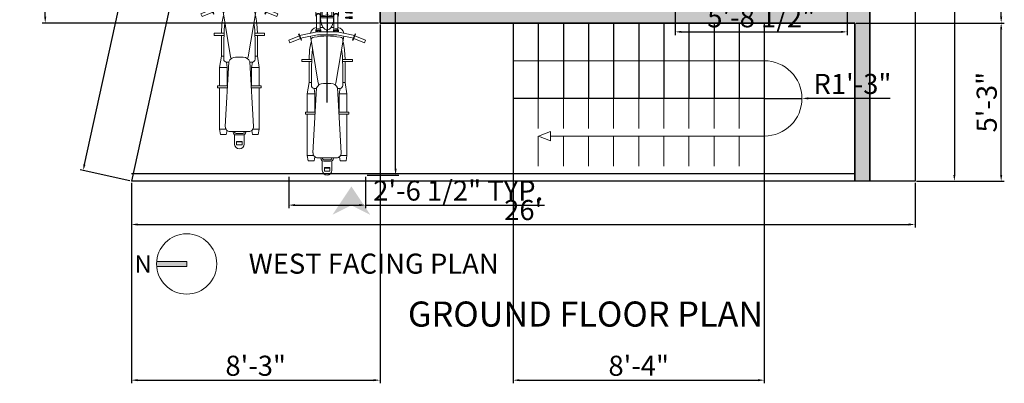
# Model space of a CAD drawing. Units: inches. Extents: x 2642 to 4124, y 1227 to 1973.
# Tile 1 of 7: x 3343 to 3735, y 1227 to 1372. Entities that reach past the tile are written whole.
import ezdxf

# ---------------------------------------------------------------- set-up
doc = ezdxf.new("R2010")
doc.units = ezdxf.units.IN
doc.linetypes.add('ACAD_ISO02W100', pattern=[15, 12, -3])
for name, color, linetype, lineweight in [('A-ANNO-DIMS', 2, 'Continuous', 18), ('A-ANNO-SYMB', 1, 'Continuous', 18), ('A-ANNO-TITL', 7, 'Continuous', 25), ('A-FLOR-STRS', 7, 'Continuous', 25), ('A-FLOR-STRS-OVHD', 7, 'ACAD_ISO02W100', 18), ('A-WALL', 7, 'Continuous', 35), ('A-WALL-PATT', 7, 'Continuous', 13), ('C-PRKG-VEHI', 8, 'Continuous', 18), ('C-PROP', 7, 'Continuous', 25)]:
    doc.layers.add(name, color=color, linetype=linetype, lineweight=lineweight)
doc.styles.get("Standard").update_dxf_attribs({"font": 'arial.ttf'})
doc.dimstyles.new('ISO-25', dxfattribs={"dimtxt": 8, "dimasz": 2.5, "dimexe": 1.25, "dimexo": 0.625, "dimtad": 1, "dimdec": 0, "dimlunit": 3, "dimtxsty": 'Standard', "dimcen": 2.5, "dimadec": 0, "dimazin": 0, "dimtfac": 1, "dimtdec": 0, "dimtmove": 0, "dimatfit": 3, "dimfxl": 1, "dimarcsym": 0})

# ---------------------------------------------------------------- blocks, each defined once
blk = doc.blocks.new('*D2')
at = {"layer": 'A-ANNO-DIMS', "color": 0, "lineweight": -2, "transparency": 16777216}
for p, q in [((3699.85, 1907.78), (3716.14, 1907.78)), ((3714.89, 1905.28), (3714.89, 1310.28)), ((3699.85, 1307.78), (3716.14, 1307.78))]:
    blk.add_line(p, q, dxfattribs=at)
at = {"layer": 'A-ANNO-DIMS', "color": 0, "transparency": 16777216}
for points in [[(3714.47, 1905.28), (3715.3, 1905.28), (3714.89, 1907.78)], [(3714.47, 1310.28), (3715.3, 1310.28), (3714.89, 1307.78)]]:
    blk.add_solid(points, dxfattribs=at)
at = {"layer": 'Defpoints', "color": 0, "transparency": 16777216}
for p in [(3699.22, 1907.78), (3699.22, 1307.78), (3714.89, 1307.78)]:
    blk.add_point(p, dxfattribs=at)
at = {"layer": 'A-ANNO-DIMS', "color": 0, "transparency": 16777216, "insert": (3710.18, 1607.78), "char_height": 8, "attachment_point": 5, "rotation": 90}
blk.add_mtext("50'", dxfattribs=at)
blk = doc.blocks.new('*D3')
at = {"layer": 'A-ANNO-DIMS', "color": 0, "lineweight": -2, "transparency": 16777216}
for p, q in [((3387.22, 1307.16), (3387.22, 1289.31)), ((3699.22, 1307.16), (3699.22, 1289.31)), ((3389.72, 1290.56), (3696.72, 1290.56))]:
    blk.add_line(p, q, dxfattribs=at)
at = {"layer": 'A-ANNO-DIMS', "color": 0, "transparency": 16777216}
for points in [[(3389.72, 1290.98), (3389.72, 1290.14), (3387.22, 1290.56)], [(3696.72, 1290.98), (3696.72, 1290.14), (3699.22, 1290.56)]]:
    blk.add_solid(points, dxfattribs=at)
at = {"layer": 'Defpoints', "color": 0, "transparency": 16777216}
for p in [(3387.22, 1307.78), (3699.22, 1307.78), (3699.22, 1290.56)]:
    blk.add_point(p, dxfattribs=at)
at = {"layer": 'A-ANNO-DIMS', "color": 0, "transparency": 16777216, "insert": (3543.22, 1295.27), "char_height": 8, "attachment_point": 5}
blk.add_mtext("26'", dxfattribs=at)
blk = doc.blocks.new('*D4')
at = {"layer": 'A-ANNO-DIMS', "color": 0, "lineweight": -2, "transparency": 16777216}
for p, q in [((3368.56, 1314.45), (3499.49, 1909.57)), ((3518.61, 1907.92), (3498.8, 1912.28)), ((3386.61, 1307.92), (3366.8, 1312.28))]:
    blk.add_line(p, q, dxfattribs=at)
at = {"layer": 'A-ANNO-DIMS', "color": 0, "transparency": 16777216}
for points in [[(3499.08, 1909.65), (3499.89, 1909.48), (3500.02, 1912.01)], [(3368.15, 1314.54), (3368.97, 1314.36), (3368.02, 1312.01)]]:
    blk.add_solid(points, dxfattribs=at)
at = {"layer": 'Defpoints', "color": 0, "transparency": 16777216}
for p in [(3500.02, 1912.01), (3519.22, 1907.78), (3387.22, 1307.78)]:
    blk.add_point(p, dxfattribs=at)
at = {"layer": 'A-ANNO-DIMS', "color": 0, "transparency": 16777216, "insert": (3429.42, 1613.02), "char_height": 8, "attachment_point": 5, "rotation": 77.5926}
blk.add_mtext('51\'-2"', dxfattribs=at)
blk = doc.blocks.new('BIKE')
for p, q in [((34846.04, 15170.34), (34846.04, 15168.87)), ((34847.86, 15170.34), (34847.86, 15168.87)), ((34845.81, 15167.86), (34845.81, 15160.7)), ((34845.81, 15167.86), (34845.81, 15160.7)), ((34848.09, 15167.86), (34848.09, 15160.7)), ((34844.29, 15164.4), (34844.29, 15160.81)), ((34845.43, 15164.4), (34845.43, 15160.81)), ((34845.43, 15164.1), (34845.81, 15164.1)), ((34845.43, 15163.85), (34845.81, 15163.85)), ((34848.47, 15164.1), (34848.09, 15164.1)), ((34848.47, 15163.85), (34848.09, 15163.85)), ((34848.47, 15164.4), (34848.47, 15160.81)), ((34849.61, 15164.4), (34849.61, 15160.81)), ((34844.41, 15160.81), (34844.41, 15157.43)), ((34845.32, 15160.81), (34845.32, 15157.43)), ((34848.58, 15160.81), (34848.58, 15157.43)), ((34849.5, 15160.81), (34849.5, 15157.43)), ((34848.51, 15160.53), (34845.39, 15160.53)), ((34845.39, 15160.23), (34845.39, 15160.53)), ((34845.39, 15160.23), (34845.39, 15160.53)), ((34848.51, 15160.23), (34845.39, 15160.23)), ((34848.51, 15160.23), (34848.51, 15160.53)), ((34840.19, 15156.35), (34840.3, 15156.39)), ((34840.19, 15156.35), (34840.8, 15154.88)), ((34840.3, 15156.39), (34840.9, 15154.92)), ((34840.47, 15155.97), (34840.8, 15156.11)), ((34840.8, 15156.11), (34844.56, 15156.88)), ((34841, 15155.45), (34844.63, 15156.2)), ((34844.29, 15156.87), (34844.29, 15157.17)), ((34844.41, 15156.87), (34844.41, 15156.85)), ((34844.56, 15156.88), (34846.95, 15156.88)), ((34844.63, 15156.2), (34846.95, 15156.2)), ((34845.32, 15157.92), (34846.04, 15157.92)), ((34845.43, 15156.87), (34845.43, 15157.17)), ((34849.34, 15156.88), (34846.95, 15156.88)), ((34849.27, 15156.2), (34846.95, 15156.2)), ((34848.58, 15157.92), (34847.87, 15157.92)), ((34848.47, 15156.87), (34848.47, 15157.17)), ((34852.9, 15155.45), (34849.27, 15156.2)), ((34853.1, 15156.11), (34849.34, 15156.88)), ((34849.5, 15156.87), (34849.5, 15156.85)), ((34849.61, 15156.87), (34849.61, 15157.17)), ((34853.6, 15156.39), (34853, 15154.92)), ((34853.71, 15156.35), (34853.1, 15154.88)), ((34853.43, 15155.97), (34853.1, 15156.11)), ((34853.71, 15156.35), (34853.6, 15156.39)), ((34837.84, 15154.89), (34840.37, 15155.93)), ((34837.84, 15154.89), (34838.1, 15154.26)), ((34838.1, 15154.26), (34840.63, 15155.3)), ((34840.73, 15155.34), (34841, 15155.45)), ((34840.8, 15154.88), (34840.9, 15154.92)), ((34842.8, 15152.59), (34843.06, 15154.2)), ((34844.86, 15144.72), (34843.01, 15155.87)), ((34843.06, 15154.2), (34843.22, 15154.58)), ((34849.05, 15144.72), (34850.89, 15155.87)), ((34850.84, 15154.2), (34850.68, 15154.58)), ((34851.1, 15152.59), (34850.84, 15154.2)), ((34853.17, 15155.34), (34852.9, 15155.45)), ((34853.1, 15154.88), (34853, 15154.92)), ((34855.81, 15154.26), (34853.28, 15155.3)), ((34856.07, 15154.89), (34853.54, 15155.93)), ((34856.07, 15154.89), (34855.81, 15154.26)), ((34842.7, 15150.31), (34842.8, 15152.59)), ((34843.33, 15151.09), (34843.52, 15152.8)), ((34850.57, 15151.09), (34850.38, 15152.8)), ((34851.2, 15150.31), (34851.1, 15152.59)), ((34840.97, 15150.31), (34843.3, 15150.31)), ((34840.97, 15149.81), (34840.97, 15150.31)), ((34843.29, 15149.81), (34840.97, 15149.81)), ((34842.7, 15144.87), (34842.7, 15149.81)), ((34843.23, 15147.75), (34843.33, 15151.09)), ((34850.67, 15147.75), (34850.57, 15151.09)), ((34852.93, 15150.31), (34850.6, 15150.31)), ((34850.61, 15149.81), (34852.93, 15149.81)), ((34851.2, 15144.87), (34851.2, 15149.81)), ((34852.93, 15149.81), (34852.93, 15150.31)), ((34843.23, 15144.15), (34843.23, 15147.75)), ((34850.67, 15144.15), (34850.67, 15147.75)), ((34842.7, 15144.87), (34842.25, 15142.19)), ((34842.7, 15144.87), (34843.23, 15144.87)), ((34847.85, 15144.64), (34846.06, 15144.64)), ((34851.2, 15144.87), (34850.67, 15144.87)), ((34851.2, 15144.87), (34851.65, 15142.19)), ((34842.25, 15142.19), (34844.07, 15142.19)), ((34842.25, 15137.82), (34842.25, 15142.19)), ((34844.46, 15143.56), (34843.6, 15128.2)), ((34843.85, 15143.46), (34844.07, 15142.19)), ((34843.91, 15143.46), (34844.46, 15143.46)), ((34844.07, 15137.82), (34844.07, 15142.19)), ((34849.44, 15143.56), (34850.3, 15128.2)), ((34849.99, 15143.46), (34849.44, 15143.46)), ((34850.05, 15143.46), (34849.83, 15142.19)), ((34851.65, 15142.19), (34849.83, 15142.19)), ((34849.83, 15137.82), (34849.83, 15142.19)), ((34851.65, 15137.82), (34851.65, 15142.19)), ((34841.79, 15137.82), (34844.14, 15137.82)), ((34841.79, 15137.33), (34841.79, 15137.82)), ((34852.11, 15137.82), (34849.76, 15137.82)), ((34852.11, 15137.33), (34852.11, 15137.82)), ((34844.11, 15137.33), (34841.79, 15137.33)), ((34842.25, 15127.57), (34842.25, 15137.33)), ((34844.07, 15136.55), (34844.07, 15137.33)), ((34849.79, 15137.33), (34852.11, 15137.33)), ((34849.83, 15136.55), (34849.83, 15137.33)), ((34851.65, 15127.57), (34851.65, 15137.33)), ((34842.25, 15127.57), (34843.75, 15127.57)), ((34842.25, 15127.57), (34842.48, 15126.27)), ((34842.48, 15126.27), (34843.84, 15126.27)), ((34844.02, 15127.25), (34843.84, 15126.27)), ((34849.16, 15126.99), (34844.74, 15126.99)), ((34845.47, 15126.99), (34845.47, 15126.88)), ((34845.81, 15126.99), (34845.81, 15126.88)), ((34845.81, 15126.29), (34845.81, 15124.03)), ((34847.75, 15126.54), (34846.15, 15126.54)), ((34847.75, 15126.2), (34846.15, 15126.2)), ((34848.09, 15126.99), (34848.09, 15126.88)), ((34848.09, 15126.29), (34848.09, 15124.03)), ((34848.43, 15126.99), (34848.43, 15126.88)), ((34849.89, 15127.25), (34850.06, 15126.27)), ((34851.43, 15126.27), (34850.06, 15126.27)), ((34851.65, 15127.57), (34850.15, 15127.57)), ((34851.65, 15127.57), (34851.43, 15126.27)), ((34846.29, 15123.82), (34846.29, 15124.66)), ((34846.29, 15124.66), (34847.61, 15124.66)), ((34846.29, 15124.55), (34847.61, 15124.55)), ((34847.61, 15123.82), (34846.29, 15123.82)), ((34847.61, 15124.66), (34847.61, 15123.82))]:
    blk.add_line(p, q)
for points in [[(34845.81, 15167.86, -0.068977), (34845.9, 15168.53, -0.081012), (34846.15, 15169.05, -0.107014), (34846.54, 15169.42, -0.137239), (34846.95, 15169.53, -0.137239), (34847.36, 15169.42, -0.107014), (34847.76, 15169.05, -0.081012), (34848, 15168.53, -0.068977), (34848.09, 15167.86, -0.068977)], [(34845.43, 15164.4, 0.125099), (34845.39, 15164.56, 0.105827), (34845.27, 15164.71, 0.086577), (34845.09, 15164.8, 0.0766), (34844.86, 15164.84, 0.0766), (34844.64, 15164.8, 0.086577), (34844.46, 15164.71, 0.105827), (34844.33, 15164.56, 0.125099), (34844.29, 15164.4, 0.125099)], [(34848.47, 15164.4, -0.125099), (34848.51, 15164.56, -0.105827), (34848.64, 15164.71, -0.086577), (34848.82, 15164.8, -0.0766), (34849.04, 15164.84, -0.0766), (34849.26, 15164.8, -0.086577), (34849.44, 15164.71, -0.105827), (34849.57, 15164.56, -0.125099), (34849.61, 15164.4, -0.125099)], [(34845.32, 15160.55, 0.067261), (34845.39, 15160.65, 0.125099), (34845.43, 15160.81, 0.125099), (34845.39, 15160.97, 0.105827), (34845.27, 15161.12, 0.086577), (34845.09, 15161.21, 0.0766), (34844.86, 15161.25, 0.0766), (34844.64, 15161.21, 0.086577), (34844.46, 15161.12, 0.105827), (34844.33, 15160.97, 0.125099), (34844.29, 15160.81, 0.125099)], [(34844.29, 15160.81, 0.125099), (34844.33, 15160.65, 0.067261), (34844.41, 15160.55, 0.086577)], [(34845.32, 15160.81, 0.125099), (34845.29, 15160.92, 0.105827), (34845.2, 15161.03, 0.086577), (34845.05, 15161.1, 0.0766), (34844.86, 15161.13, 0.0766), (34844.67, 15161.1, 0.086577), (34844.53, 15161.03, 0.105827), (34844.43, 15160.92, 0.125099), (34844.41, 15160.81, 0.125099)], [(34848.58, 15160.55, -0.067261), (34848.51, 15160.65, -0.125099), (34848.47, 15160.81, -0.125099), (34848.51, 15160.97, -0.105827), (34848.64, 15161.12, -0.086577), (34848.82, 15161.21, -0.0766), (34849.04, 15161.25, -0.0766), (34849.26, 15161.21, -0.086577), (34849.44, 15161.12, -0.105827), (34849.57, 15160.97, -0.125099), (34849.61, 15160.81, -0.125099)], [(34848.58, 15160.81, -0.125099), (34848.61, 15160.92, -0.105827), (34848.71, 15161.03, -0.086577), (34848.85, 15161.1, -0.0766), (34849.04, 15161.13, -0.0766), (34849.23, 15161.1, -0.086577), (34849.37, 15161.03, -0.105827), (34849.47, 15160.92, -0.125099), (34849.5, 15160.81, -0.125099)], [(34849.61, 15160.81, -0.125099), (34849.57, 15160.65, -0.067261), (34849.5, 15160.55, -0.086577)], [(34846.95, 15157.37, -0.163989), (34846.41, 15157.55, -0.105862), (34845.85, 15158.21, -0.069323), (34845.52, 15159.08, -0.055531), (34845.39, 15160.23, -0.055531)], [(34848.51, 15160.23, -0.055531), (34848.38, 15159.08, -0.069323), (34848.06, 15158.21, -0.105862), (34847.49, 15157.55, -0.163989), (34846.95, 15157.37, -0.163989)], [(34845.43, 15157.17, 0.125099), (34845.39, 15157.33, 0.105827), (34845.27, 15157.48, 0.086577), (34845.09, 15157.57, 0.0766), (34844.86, 15157.6, 0.0766), (34844.64, 15157.57, 0.086577), (34844.46, 15157.48, 0.105827), (34844.33, 15157.33, 0.125099), (34844.29, 15157.17, 0.125099)], [(34845.43, 15156.88, 0.117252), (34845.39, 15157.03, 0.105827), (34845.27, 15157.18, 0.086577), (34845.09, 15157.27, 0.0766), (34844.86, 15157.31, 0.0766), (34844.64, 15157.27, 0.086577), (34844.46, 15157.18, 0.105827), (34844.33, 15157.03, 0.125099), (34844.29, 15156.87, 0.125099)], [(34844.29, 15156.87, 0.032819), (34844.3, 15156.83, 0.067261)], [(34845.32, 15156.88, 0.113202), (34845.29, 15156.98, 0.105827), (34845.2, 15157.09, 0.086577), (34845.05, 15157.16, 0.0766), (34844.86, 15157.19, 0.0766), (34844.67, 15157.16, 0.086577), (34844.53, 15157.09, 0.105827), (34844.43, 15156.98, 0.125099), (34844.41, 15156.87, 0.125099)], [(34848.47, 15157.17, -0.125099), (34848.51, 15157.33, -0.105827), (34848.64, 15157.48, -0.086577), (34848.82, 15157.57, -0.0766), (34849.04, 15157.6, -0.0766), (34849.26, 15157.57, -0.086577), (34849.44, 15157.48, -0.105827), (34849.57, 15157.33, -0.125099), (34849.61, 15157.17, -0.125099)], [(34848.47, 15156.88, -0.117252), (34848.51, 15157.03, -0.105827), (34848.64, 15157.18, -0.086577), (34848.82, 15157.27, -0.0766), (34849.04, 15157.31, -0.0766), (34849.26, 15157.27, -0.086577), (34849.44, 15157.18, -0.105827), (34849.57, 15157.03, -0.125099), (34849.61, 15156.87, -0.125099)], [(34848.58, 15156.88, -0.113202), (34848.61, 15156.98, -0.105827), (34848.71, 15157.09, -0.086577), (34848.85, 15157.16, -0.0766), (34849.04, 15157.19, -0.0766), (34849.23, 15157.16, -0.086577), (34849.37, 15157.09, -0.105827), (34849.47, 15156.98, -0.125099), (34849.5, 15156.87, -0.125099)], [(34849.61, 15156.87, -0.032819), (34849.61, 15156.83, -0.067261)]]:
    blk.add_lwpolyline(points, format="xyb")
for centre, radius, start, end in [((34846.95, 15157.24), 3.64, 64.5882, 115.4118), ((34844.55, 15156.32), 1.59, 95.2207, 171.678), ((34849.35, 15156.32), 1.59, 8.322, 84.7793), ((34843.86, 15154.92), 0.684, 90, 189.3898), ((34846.95, 15140.12), 15.79, 78.7129, 101.2871), ((34850.04, 15154.92), 0.684, 350.6102, 90), ((34846, 15143), 1.64, 88.1125, 159.9264), ((34845.53, 15144.83), 0.684, 189.3898, 226.4877), ((34847.9, 15143), 1.64, 20.0736, 91.8875), ((34848.37, 15144.83), 0.684, 313.5123, 350.6102), ((34843.91, 15144.15), 0.684, 180, 270), ((34849.99, 15144.15), 0.684, 270, 0), ((34844.74, 15128.13), 1.14, 176.7865, 270), ((34849.16, 15128.13), 1.14, 270, 3.2135), ((34846.15, 15126.88), 0.684, 180, 270), ((34846.15, 15126.88), 0.342, 180, 270), ((34847.75, 15126.88), 0.684, 270, 0), ((34847.75, 15126.88), 0.342, 270, 0), ((34846.95, 15124.03), 1.14, 180, 0)]:
    blk.add_arc(centre, radius, start, end)
blk = doc.blocks.new('*D48')
at = {"layer": 'A-ANNO-DIMS', "color": 0, "lineweight": -2, "transparency": 16777216}
for p, q in [((3492.41, 1389.89), (3492.41, 1489.27)), ((3481.09, 1389.89), (3493.66, 1389.89)), ((3492.41, 1312.73), (3492.41, 1387.39)), ((3481.09, 1310.23), (3493.66, 1310.23))]:
    blk.add_line(p, q, dxfattribs=at)
at = {"layer": 'A-ANNO-DIMS', "color": 0, "transparency": 16777216}
for points in [[(3492, 1387.39), (3492.83, 1387.39), (3492.41, 1389.89)], [(3492, 1312.73), (3492.83, 1312.73), (3492.41, 1310.23)]]:
    blk.add_solid(points, dxfattribs=at)
at = {"layer": 'Defpoints', "color": 0, "transparency": 16777216}
for p in [(3480.46, 1389.89), (3492.41, 1389.89), (3480.46, 1310.23)]:
    blk.add_point(p, dxfattribs=at)
at = {"layer": 'A-ANNO-DIMS', "color": 0, "transparency": 16777216, "insert": (3487.65, 1440.83), "char_height": 8, "attachment_point": 5, "rotation": 90}
blk.add_mtext('BIKE 6\'-7 1/2" TYP.', dxfattribs=at)
blk = doc.blocks.new('*D49')
at = {"layer": 'A-ANNO-DIMS', "color": 0, "lineweight": -2, "transparency": 16777216}
for p, q in [((3449.86, 1309.6), (3449.86, 1297.03)), ((3480.46, 1309.6), (3480.46, 1297.03)), ((3452.36, 1298.28), (3477.96, 1298.28)), ((3480.46, 1298.28), (3551.75, 1298.28))]:
    blk.add_line(p, q, dxfattribs=at)
at = {"layer": 'A-ANNO-DIMS', "color": 0, "transparency": 16777216}
for points in [[(3452.36, 1298.69), (3452.36, 1297.86), (3449.86, 1298.28)], [(3477.96, 1298.69), (3477.96, 1297.86), (3480.46, 1298.28)]]:
    blk.add_solid(points, dxfattribs=at)
at = {"layer": 'Defpoints', "color": 0, "transparency": 16777216}
for p in [(3449.86, 1310.23), (3480.46, 1310.23), (3480.46, 1298.28)]:
    blk.add_point(p, dxfattribs=at)
at = {"layer": 'A-ANNO-DIMS', "color": 0, "transparency": 16777216, "insert": (3517.36, 1303.04), "char_height": 8, "attachment_point": 5}
blk.add_mtext('2\'-6 1/2" TYP.', dxfattribs=at)
blk = doc.blocks.new('*D55')
at = {"layer": 'A-ANNO-DIMS', "color": 0, "lineweight": -2, "transparency": 16777216}
for p, q in [((3603.75, 1379.31), (3603.75, 1366.03)), ((3672.22, 1379.31), (3672.22, 1366.03)), ((3606.25, 1367.28), (3669.72, 1367.28))]:
    blk.add_line(p, q, dxfattribs=at)
at = {"layer": 'A-ANNO-DIMS', "color": 0, "transparency": 16777216}
for points in [[(3606.25, 1367.7), (3606.25, 1366.87), (3603.75, 1367.28)], [(3669.72, 1367.7), (3669.72, 1366.87), (3672.22, 1367.28)]]:
    blk.add_solid(points, dxfattribs=at)
at = {"layer": 'Defpoints', "color": 0, "transparency": 16777216}
for p in [(3603.75, 1379.93), (3672.22, 1379.93), (3672.22, 1367.28)]:
    blk.add_point(p, dxfattribs=at)
at = {"layer": 'A-ANNO-DIMS', "color": 0, "transparency": 16777216, "insert": (3637.99, 1372.04), "char_height": 8, "attachment_point": 5}
blk.add_mtext('5\'-8 1/2"', dxfattribs=at)
blk = doc.blocks.new('*D68')
at = {"layer": 'A-ANNO-DIMS', "color": 0, "lineweight": -2, "transparency": 16777216}
for p, q in [((3675.85, 1370.78), (3734.77, 1370.78)), ((3733.52, 1310.28), (3733.52, 1368.28)), ((3699.85, 1307.78), (3734.77, 1307.78))]:
    blk.add_line(p, q, dxfattribs=at)
at = {"layer": 'A-ANNO-DIMS', "color": 0, "transparency": 16777216}
for points in [[(3733.11, 1368.28), (3733.94, 1368.28), (3733.52, 1370.78)], [(3733.11, 1310.28), (3733.94, 1310.28), (3733.52, 1307.78)]]:
    blk.add_solid(points, dxfattribs=at)
at = {"layer": 'Defpoints', "color": 0, "transparency": 16777216}
for p in [(3675.22, 1370.78), (3733.52, 1370.78), (3699.22, 1307.78)]:
    blk.add_point(p, dxfattribs=at)
at = {"layer": 'A-ANNO-DIMS', "color": 0, "transparency": 16777216, "insert": (3728.81, 1339.28), "char_height": 8, "attachment_point": 5, "rotation": 90}
blk.add_mtext('5\'-3"', dxfattribs=at)
blk = doc.blocks.new('*D69')
at = {"layer": 'A-ANNO-DIMS', "color": 0, "lineweight": -2, "transparency": 16777216}
for p, q in [((3486.22, 1370.16), (3486.22, 1227.29)), ((3387.22, 1307.16), (3387.22, 1227.29)), ((3389.72, 1228.54), (3483.72, 1228.54))]:
    blk.add_line(p, q, dxfattribs=at)
at = {"layer": 'A-ANNO-DIMS', "color": 0, "transparency": 16777216}
for points in [[(3389.72, 1228.96), (3389.72, 1228.12), (3387.22, 1228.54)], [(3483.72, 1228.96), (3483.72, 1228.12), (3486.22, 1228.54)]]:
    blk.add_solid(points, dxfattribs=at)
at = {"layer": 'Defpoints', "color": 0, "transparency": 16777216}
for p in [(3486.22, 1370.78), (3387.22, 1307.78), (3486.22, 1228.54)]:
    blk.add_point(p, dxfattribs=at)
at = {"layer": 'A-ANNO-DIMS', "color": 0, "transparency": 16777216, "insert": (3436.72, 1233.25), "char_height": 8, "attachment_point": 5}
blk.add_mtext('8\'-3"', dxfattribs=at)
blk = doc.blocks.new('*D72')
at = {"layer": 'A-ANNO-DIMS', "color": 0, "lineweight": -2, "transparency": 16777216}
for p, q in [((3485.6, 1508.78), (3351.67, 1508.78)), ((3352.92, 1373.28), (3352.92, 1506.28)), ((3485.6, 1370.78), (3351.67, 1370.78))]:
    blk.add_line(p, q, dxfattribs=at)
at = {"layer": 'A-ANNO-DIMS', "color": 0, "transparency": 16777216}
for points in [[(3352.51, 1506.28), (3353.34, 1506.28), (3352.92, 1508.78)], [(3352.51, 1373.28), (3353.34, 1373.28), (3352.92, 1370.78)]]:
    blk.add_solid(points, dxfattribs=at)
at = {"layer": 'Defpoints', "color": 0, "transparency": 16777216}
for p in [(3352.92, 1508.78), (3486.22, 1508.78), (3486.22, 1370.78)]:
    blk.add_point(p, dxfattribs=at)
at = {"layer": 'A-ANNO-DIMS', "color": 0, "transparency": 16777216, "insert": (3348.21, 1439.78), "char_height": 8, "attachment_point": 5, "rotation": 90}
blk.add_mtext('11\'-6"', dxfattribs=at)
blk = doc.blocks.new('*D73')
at = {"layer": 'A-ANNO-DIMS', "color": 0, "lineweight": -2, "transparency": 16777216}
for p, q in [((3539.22, 1370.16), (3539.22, 1227.29)), ((3639.22, 1370.16), (3639.22, 1227.29)), ((3541.72, 1228.54), (3636.72, 1228.54))]:
    blk.add_line(p, q, dxfattribs=at)
at = {"layer": 'A-ANNO-DIMS', "color": 0, "transparency": 16777216}
for points in [[(3541.72, 1228.96), (3541.72, 1228.12), (3539.22, 1228.54)], [(3636.72, 1228.96), (3636.72, 1228.12), (3639.22, 1228.54)]]:
    blk.add_solid(points, dxfattribs=at)
at = {"layer": 'Defpoints', "color": 0, "transparency": 16777216}
for p in [(3539.22, 1370.78), (3639.22, 1370.78), (3639.22, 1228.54)]:
    blk.add_point(p, dxfattribs=at)
at = {"layer": 'A-ANNO-DIMS', "color": 0, "transparency": 16777216, "insert": (3589.22, 1233.25), "char_height": 8, "attachment_point": 5}
blk.add_mtext('8\'-4"', dxfattribs=at)
blk = doc.blocks.new('*D74')
at = {"layer": 'A-ANNO-DIMS', "color": 0, "lineweight": -2, "transparency": 16777216}
for p, q in [((3681.85, 1427.78), (3734.77, 1427.78)), ((3733.52, 1373.28), (3733.52, 1425.28)), ((3675.85, 1370.78), (3734.77, 1370.78))]:
    blk.add_line(p, q, dxfattribs=at)
at = {"layer": 'A-ANNO-DIMS', "color": 0, "transparency": 16777216}
for points in [[(3733.11, 1425.28), (3733.94, 1425.28), (3733.52, 1427.78)], [(3733.11, 1373.28), (3733.94, 1373.28), (3733.52, 1370.78)]]:
    blk.add_solid(points, dxfattribs=at)
at = {"layer": 'Defpoints', "color": 0, "transparency": 16777216}
for p in [(3681.22, 1427.78), (3733.52, 1427.78), (3675.22, 1370.78)]:
    blk.add_point(p, dxfattribs=at)
at = {"layer": 'A-ANNO-DIMS', "color": 0, "transparency": 16777216, "insert": (3728.81, 1399.28), "char_height": 8, "attachment_point": 5, "rotation": 90}
blk.add_mtext('4\'-9"', dxfattribs=at)
blk = doc.blocks.new('*D82')
at = {"layer": 'A-ANNO-DIMS', "color": 0, "lineweight": -2, "transparency": 16777216}
for p, q in [((3639.22, 1340.78), (3654.22, 1340.78)), ((3689.39, 1340.78), (3656.72, 1340.78))]:
    blk.add_line(p, q, dxfattribs=at)
at = {"layer": 'A-ANNO-DIMS', "color": 0, "transparency": 16777216}
blk.add_solid([(3656.72, 1341.2), (3656.72, 1340.37), (3654.22, 1340.78)], dxfattribs=at)
at = {"layer": 'Defpoints', "color": 0, "transparency": 16777216}
for p in [(3639.22, 1340.78), (3654.22, 1340.78)]:
    blk.add_point(p, dxfattribs=at)
at = {"layer": 'A-ANNO-DIMS', "color": 0, "transparency": 16777216, "insert": (3674.31, 1345.5), "char_height": 8, "attachment_point": 5, "rotation": 359.9998}
blk.add_mtext('R1\'-3"', dxfattribs=at)
blk = doc.blocks.new('*D84')
at = {"layer": 'A-ANNO-DIMS', "color": 0, "lineweight": -2, "transparency": 16777216}
for p, q in [((3465.16, 1436.8), (3465.16, 1368.17)), ((3465.16, 1339.16), (3465.16, 1365.67))]:
    blk.add_line(p, q, dxfattribs=at)
at = {"layer": 'A-ANNO-DIMS', "color": 0, "transparency": 16777216}
blk.add_solid([(3465.58, 1368.17), (3464.74, 1368.17), (3465.16, 1365.67)], dxfattribs=at)
at = {"layer": 'Defpoints', "color": 0, "transparency": 16777216}
for p in [(3465.16, 1365.67), (3465.16, 1339.16)]:
    blk.add_point(p, dxfattribs=at)
at = {"layer": 'A-ANNO-DIMS', "color": 0, "transparency": 16777216, "insert": (3469.92, 1403.74), "char_height": 8, "attachment_point": 5, "rotation": 270.0011}
blk.add_mtext('2X R2\'-2 1/2"', dxfattribs=at)

msp = doc.modelspace()

# ---------------------------------------------------------------- hatches: boundary and pattern name
at = {"layer": 'A-ANNO-SYMB'}
h = msp.add_hatch(color=256, dxfattribs=at)
h.dxf.hatch_style = 1
h.paths.add_polyline_path([(3474.82, 1305.73), (3467.27, 1294.41), (3474.82, 1298.18), (3482.37, 1294.41)])
h = msp.add_hatch(color=256, dxfattribs=at)
h.dxf.hatch_style = 1
h.paths.add_polyline_path([(3409.24, 1275.84), (3409.24, 1273.84), (3397.28, 1273.84, -0.020861), (3397.24, 1274.84, -0.020861), (3397.28, 1275.84)])
at = {"layer": 'A-WALL-PATT'}
h = msp.add_hatch(color=256, dxfattribs=at)
h.dxf.hatch_style = 1
h.paths.add_polyline_path([(3552.22, 1505.78), (3495.22, 1505.78), (3495.22, 1508.78), (3492.22, 1508.78), (3486.22, 1508.78), (3486.22, 1415.78), (3495.22, 1415.78), (3495.22, 1499.78), (3543.22, 1499.78), (3543.22, 1457.78), (3549.22, 1457.78), (3549.22, 1499.78), (3552.19, 1499.78), (3552.19, 1499.78)])
h.paths.add_polyline_path([(3681.22, 1427.78), (3672.22, 1427.78), (3672.22, 1395.07), (3672.22, 1379.78), (3549.22, 1379.78), (3549.22, 1427.78), (3543.22, 1427.78), (3543.22, 1379.78), (3495.22, 1379.78), (3495.22, 1391.78), (3486.22, 1391.78), (3486.22, 1370.78), (3675.22, 1370.78), (3675.22, 1307.78), (3681.22, 1307.78)])
h.paths.add_polyline_path([(3681.22, 1517.78), (3672.22, 1517.78), (3672.22, 1505.78), (3640.73, 1505.78), (3588.22, 1505.78), (3588.22, 1499.78), (3672.22, 1499.78), (3672.22, 1475.78), (3681.22, 1475.78)])
h.paths.add_polyline_path([(3681.22, 1638.12), (3672.22, 1638.12), (3672.22, 1625.78), (3681.22, 1625.78)])
h.paths.add_polyline_path([(3681.22, 1553.78), (3672.22, 1553.78), (3672.22, 1541.78), (3681.22, 1541.78)])
h.paths.add_polyline_path([(3528.22, 1844.78), (3552.22, 1844.78), (3552.22, 1847.78), (3552.22, 1853.78), (3519.22, 1853.78), (3519.22, 1682.78), (3486.22, 1682.78), (3486.22, 1548.78), (3492.22, 1548.78), (3495.22, 1548.78), (3495.22, 1673.78), (3528.22, 1673.78)])
h.paths.add_polyline_path([(3681.22, 1865.78), (3675.22, 1865.78), (3675.22, 1853.78), (3615.22, 1853.78), (3615.22, 1856.78), (3609.22, 1856.78), (3609.22, 1853.78), (3582.22, 1853.78), (3582.22, 1847.78), (3582.22, 1844.78), (3672.22, 1844.78), (3672.22, 1823.67), (3681.22, 1823.67)])
h.paths.add_polyline_path([(3681.22, 1907.78), (3519.22, 1907.78), (3519.22, 1901.78), (3540.68, 1901.78), (3609.22, 1901.78), (3609.22, 1886.78), (3615.22, 1886.78), (3615.22, 1901.78), (3675.22, 1901.78), (3675.22, 1889.78), (3681.22, 1889.78)])
h.paths.add_polyline_path([(3681.22, 1775.67), (3672.22, 1775.67), (3672.22, 1742.87), (3681.22, 1742.87)])
h.paths.add_polyline_path([(3681.22, 1694.87), (3672.22, 1694.87), (3672.22, 1682.78), (3600.22, 1682.78), (3600.22, 1673.78), (3672.22, 1673.78), (3672.22, 1662.12), (3681.22, 1662.12)])

# ---------------------------------------------------------------- linework, layer by layer
at = {"layer": 'A-ANNO-SYMB'}
for p, q in [((3409.24, 1275.84), (3397.28, 1275.84)), ((3409.24, 1273.84), (3409.24, 1275.84)), ((3397.24, 1273.84), (3409.24, 1273.84))]:
    msp.add_line(p, q, dxfattribs=at)
for points in [[(3539.22, 1355.78), (3639.22, 1355.78)], [(3554.08, 1325.78), (3639.22, 1325.78)]]:
    msp.add_lwpolyline(points, dxfattribs=at)
msp.add_lwpolyline([(3549.32, 1325.78), (3554.08, 1323.91), (3554.08, 1327.65)], close=True, dxfattribs=at)
msp.add_circle((3409.24, 1274.84), 12, dxfattribs=at)
msp.add_arc((3639.22, 1340.78), 15, 270, 90, dxfattribs=at)
at = {"layer": 'A-FLOR-STRS'}
for p, q in [((3539.22, 1370.78), (3539.22, 1340.78)), ((3549.22, 1370.78), (3549.22, 1340.78)), ((3559.22, 1370.78), (3559.22, 1340.78)), ((3569.22, 1370.78), (3569.22, 1340.78)), ((3579.22, 1370.78), (3579.22, 1340.78)), ((3589.22, 1370.78), (3589.22, 1340.78)), ((3599.22, 1370.78), (3599.22, 1340.78)), ((3609.22, 1370.78), (3609.22, 1340.78)), ((3619.22, 1370.78), (3619.22, 1340.78)), ((3629.22, 1370.78), (3629.22, 1340.78)), ((3639.22, 1370.78), (3639.22, 1310.78)), ((3639.22, 1340.78), (3539.22, 1340.78))]:
    msp.add_line(p, q, dxfattribs=at)
at = {"layer": 'A-FLOR-STRS-OVHD'}
for p, q in [((3549.22, 1340.78), (3549.22, 1310.78)), ((3559.22, 1340.78), (3559.22, 1310.78)), ((3569.22, 1340.78), (3569.22, 1310.78)), ((3579.22, 1340.78), (3579.22, 1310.78)), ((3589.22, 1340.78), (3589.22, 1310.78)), ((3599.22, 1340.78), (3599.22, 1310.78)), ((3609.22, 1340.78), (3609.22, 1310.78)), ((3619.22, 1340.78), (3619.22, 1310.78)), ((3629.22, 1340.78), (3629.22, 1310.78))]:
    msp.add_line(p, q, dxfattribs=at)
at = {"layer": 'A-WALL'}
for p, q in [((3681.22, 1907.78), (3681.22, 1307.78)), ((3486.22, 1508.78), (3486.22, 1370.78)), ((3675.22, 1370.78), (3486.22, 1370.78)), ((3675.22, 1370.78), (3675.22, 1307.78))]:
    msp.add_line(p, q, dxfattribs=at)
at = {"layer": 'C-PROP'}
for p, q in [((3519.22, 1907.78), (3387.22, 1307.78)), ((3699.22, 1907.78), (3699.22, 1307.78)), ((3675.22, 1310.78), (3387.22, 1310.78)), ((3699.22, 1307.78), (3387.22, 1307.78))]:
    msp.add_line(p, q, dxfattribs=at)

# ---------------------------------------------------------------- block references
at = {"layer": 'C-PRKG-VEHI', "xscale": 1.67889555227424, "yscale": 1.67889555227424, "zscale": 1.67889555227424}
for p in [(-55074.15, -24069.06), (-55039.23, -24079.53)]:
    msp.add_blockref('BIKE', p, dxfattribs=at)

# ---------------------------------------------------------------- texts
at = {"layer": 'A-ANNO-SYMB'}
msp.add_text('N', height=6.9, dxfattribs=at).set_placement((3388.5, 1271.31))
at = {"layer": 'A-ANNO-TITL', "attachment_point": 1}
for s, insert, char_height in [('{\\fTimes New Roman|b0|i0|c0|p18;WEST FACING PLAN}', (3433.93, 1278.96), 8), ('{\\fTimes New Roman|b0|i0|c0|p18;GROUND FLOOR PLAN}', (3497.33, 1259.88), 10)]:
    msp.add_mtext_dynamic_manual_height_columns(s, width=196.2607, gutter_width=12.5, heights=[0], dxfattribs=dict(at, insert=insert, char_height=char_height))

# ---------------------------------------------------------------- dimensions: what is measured, and where the dimension line sits
at = {"layer": 'A-ANNO-DIMS'}
dim = msp.add_aligned_dim(p1=(3387.22, 1307.78), p2=(3519.22, 1907.78), distance=19.66, dimstyle='ISO-25', override={"dimclrd": 0, "dimclre": 0, "dimclrt": 0}, dxfattribs=at)
dim.commit()
dim.dimension.update_dxf_attribs({"geometry": '*D4', "text_midpoint": (3429.42, 1613.02)})
for base, p1, p2, override, picture, middle in [((3714.89, 1307.78), (3699.22, 1907.78), (3699.22, 1307.78), {"dimclrd": 0, "dimclre": 0, "dimclrt": 0}, '*D2', (3710.18, 1607.78)), ((3352.92, 1508.78), (3486.22, 1370.78), (3486.22, 1508.78), {"dimdec": 1, "dimlfac": 1, "dimrnd": 0, "dimzin": 1, "dimdsep": 46, "dimlunit": 4, "dimfrac": 2}, '*D72', (3348.21, 1439.78)), ((3733.52, 1427.78), (3675.22, 1370.78), (3681.22, 1427.78), {"dimdec": 1, "dimlfac": 1, "dimrnd": 0, "dimzin": 1, "dimdsep": 46, "dimlunit": 4, "dimfrac": 2}, '*D74', (3728.81, 1399.28)), ((3733.52, 1370.78), (3699.22, 1307.78), (3675.22, 1370.78), {"dimdec": 1, "dimlfac": 1, "dimrnd": 0, "dimzin": 1, "dimdsep": 46, "dimlunit": 4, "dimfrac": 2}, '*D68', (3728.81, 1339.28))]:
    dim = msp.add_linear_dim(base=base, p1=p1, p2=p2, angle=90, dimstyle='ISO-25', override=override, dxfattribs=at)
    dim.commit()
    dim.dimension.update_dxf_attribs({"geometry": picture, "text_midpoint": middle})
dim = msp.add_linear_dim(base=(3492.41, 1389.89), p1=(3480.46, 1310.23), p2=(3480.46, 1389.89), angle=90, text='BIKE <> TYP.', dimstyle='ISO-25', override={"dimdec": 1, "dimlfac": 1, "dimrnd": 0, "dimzin": 1, "dimdsep": 46, "dimlunit": 4, "dimfrac": 2}, dxfattribs=at)
dim.commit()
dim.dimension.update_dxf_attribs({"geometry": '*D48', "text_midpoint": (3487.65, 1440.83)})
dim = msp.add_radius_dim(center=(3465.16, 1339.16), mpoint=(3465.16, 1365.67), text='2X <>', dimstyle='ISO-25', override={"dimdec": 1, "dimlfac": 1, "dimrnd": 0, "dimzin": 1, "dimdsep": 46, "dimlunit": 4, "dimfrac": 2}, dxfattribs=at)
dim.commit()
dim.dimension.update_dxf_attribs({"geometry": '*D84', "text_midpoint": (3469.92, 1403.74)})
for base, p1, p2, override, picture, middle in [((3672.22, 1367.28), (3603.75, 1379.93), (3672.22, 1379.93), {"dimdec": 1, "dimlfac": 1, "dimrnd": 0, "dimzin": 1, "dimdsep": 46, "dimlunit": 4, "dimfrac": 2}, '*D55', (3637.99, 1372.04)), ((3486.22, 1228.54), (3387.22, 1307.78), (3486.22, 1370.78), {"dimdec": 1, "dimlfac": 1, "dimrnd": 0, "dimzin": 1, "dimdsep": 46, "dimlunit": 4, "dimfrac": 2}, '*D69', (3436.72, 1233.25)), ((3639.22, 1228.54), (3539.22, 1370.78), (3639.22, 1370.78), {"dimdec": 1, "dimlfac": 1, "dimrnd": 0, "dimzin": 1, "dimdsep": 46, "dimlunit": 4, "dimfrac": 2}, '*D73', (3589.22, 1233.25)), ((3699.22, 1290.56), (3387.22, 1307.78), (3699.22, 1307.78), {"dimclrd": 0, "dimclre": 0, "dimclrt": 0}, '*D3', (3543.22, 1295.27))]:
    dim = msp.add_linear_dim(base=base, p1=p1, p2=p2, dimstyle='ISO-25', override=override, dxfattribs=at)
    dim.commit()
    dim.dimension.update_dxf_attribs({"geometry": picture, "text_midpoint": middle})
dim = msp.add_radius_dim(center=(3639.22, 1340.78), mpoint=(3654.22, 1340.78), dimstyle='ISO-25', override={"dimdec": 1, "dimlfac": 1, "dimrnd": 0, "dimzin": 1, "dimdsep": 46, "dimlunit": 4, "dimfrac": 2}, dxfattribs=at)
dim.commit()
dim.dimension.update_dxf_attribs({"geometry": '*D82', "text_midpoint": (3674.31, 1345.5)})
dim = msp.add_linear_dim(base=(3480.46, 1298.28), p1=(3449.86, 1310.23), p2=(3480.46, 1310.23), text='<> TYP.', dimstyle='ISO-25', override={"dimdec": 1, "dimlfac": 1, "dimrnd": 0, "dimzin": 1, "dimdsep": 46, "dimlunit": 4, "dimfrac": 2}, dxfattribs=at)
dim.commit()
dim.dimension.update_dxf_attribs({"geometry": '*D49', "text_midpoint": (3517.36, 1303.04)})

doc.saveas('drawing.dxf')
